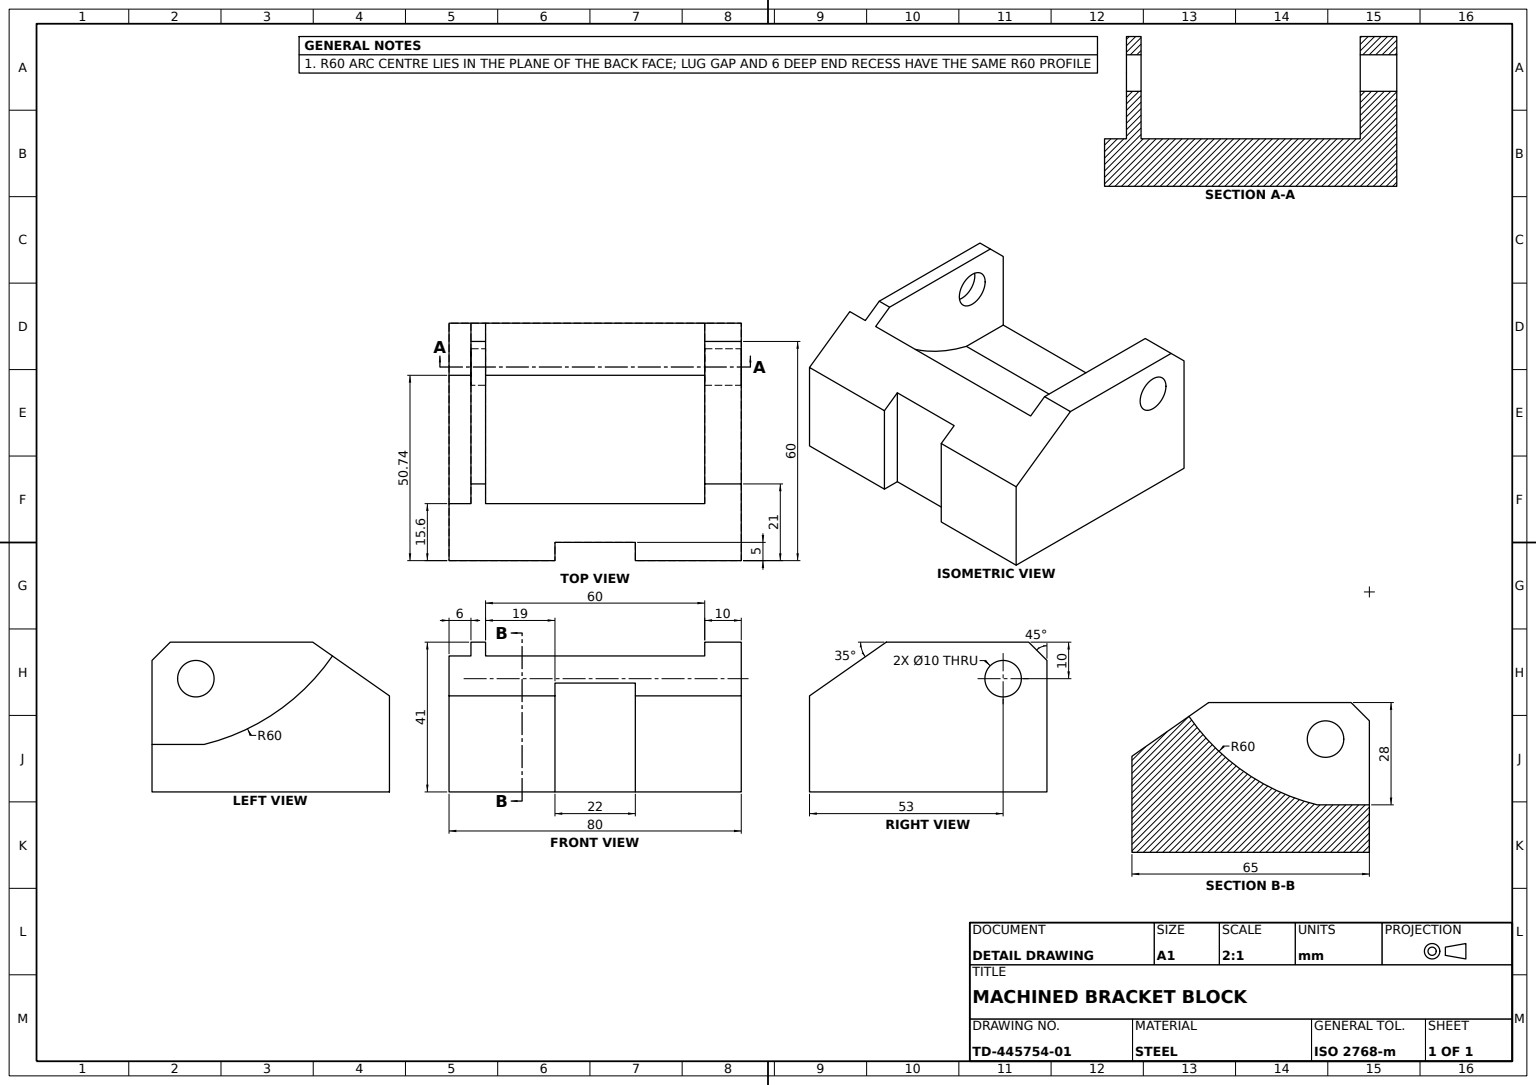
from build123d import *

# Parameters (mm, degrees)
BLOCK_PROFILE_SKETCH_W         = 65
BLOCK_PROFILE_SKETCH_H         = 41
BLOCK_PROFILE_SKETCH_R         = 5
BLOCK_BODY_80MM_DEPTH          = 40
EDGE_CHAMFER_5MM_SIZE          = 5
TOP_CHAMFER_21MM_X_35DEG_SIZE  = 21
TOP_CHAMFER_21MM_X_35DEG_SIZE2 = 14.704358302
TOP_RECESS_CUT_6MM_DEPTH       = 6
LUG_GAP_CUT_60MM_DEPTH         = 60
THROUGH_SLOT_SKETCH_W          = 5
THROUGH_SLOT_SKETCH_H          = 22
THROUGH_SLOT_CUT_DEPTH         = 210


with BuildPart() as part:
    # Block Profile Sketch → Block Body 80mm (new, symmetric)
    with BuildSketch(Plane.XY):
        with Locations((32.5, 20.5)):
            Rectangle(BLOCK_PROFILE_SKETCH_W, BLOCK_PROFILE_SKETCH_H)
        with Locations((12, 31)):
            Circle(BLOCK_PROFILE_SKETCH_R, mode=Mode.SUBTRACT)
    extrude(amount=BLOCK_BODY_80MM_DEPTH, both=True)

    # Edge Chamfer 5mm
    edge_chamfer_5mm_edges = [part.edges().sort_by_distance(p)[0] for p in [
        (0, 41, 0),
    ]]
    chamfer(edge_chamfer_5mm_edges, length=EDGE_CHAMFER_5MM_SIZE)

    # Top Chamfer 21mm x 35deg
    top_chamfer_21mm_x_35deg_edges = [part.edges().sort_by_distance(p)[0] for p in [
        (65, 41, 0),
    ]]
    top_chamfer_21mm_x_35deg_side = [part.faces().sort_by_distance(p)[0] for p in [
        (35, 41, 0),
    ]]
    chamfer(top_chamfer_21mm_x_35deg_edges, length=TOP_CHAMFER_21MM_X_35DEG_SIZE, length2=TOP_CHAMFER_21MM_X_35DEG_SIZE2, reference=top_chamfer_21mm_x_35deg_side[0])

    # Top Recess Sketch → Top Recess Cut 6mm (cut)
    with BuildSketch(Plane.XY.offset(40)):
        with BuildLine():
            Line((0, 13), (14.264629746, 13))
            ThreePointArc((14.264629746, 13), (34.056650789, 21.881854304), (49.396602602, 37.221258177))
            Line((49.396602602, 37.221258177), (44, 41))
            Line((44, 41), (5, 41))
            Line((5, 41), (0, 36))
            Line((0, 36), (0, 13))
        make_face()
    extrude(amount=-TOP_RECESS_CUT_6MM_DEPTH, mode=Mode.SUBTRACT)

    # Lug Gap Sketch → Lug Gap Cut 60mm (cut)
    with BuildSketch(Plane.XY.offset(30)):
        with BuildLine():
            Line((0, 13), (0, 36))
            Line((0, 36), (5, 41))
            Line((5, 41), (44, 41))
            Line((44, 41), (49.396602602, 37.221258177))
            ThreePointArc((49.396602602, 37.221258177), (34.056650789, 21.881854304), (14.264629746, 13))
            Line((14.264629746, 13), (0, 13))
        make_face()
    extrude(amount=-LUG_GAP_CUT_60MM_DEPTH, mode=Mode.SUBTRACT)

    # Through Slot Sketch → Through Slot Cut (cut)
    with BuildSketch(Plane(origin=(0, 41, 0), x_dir=(1, 0, 0), z_dir=(0, 1, 0))):
        with Locations((62.5, 0)):
            Rectangle(THROUGH_SLOT_SKETCH_W, THROUGH_SLOT_SKETCH_H)
    extrude(amount=-THROUGH_SLOT_CUT_DEPTH, mode=Mode.SUBTRACT)


solid = part.part
